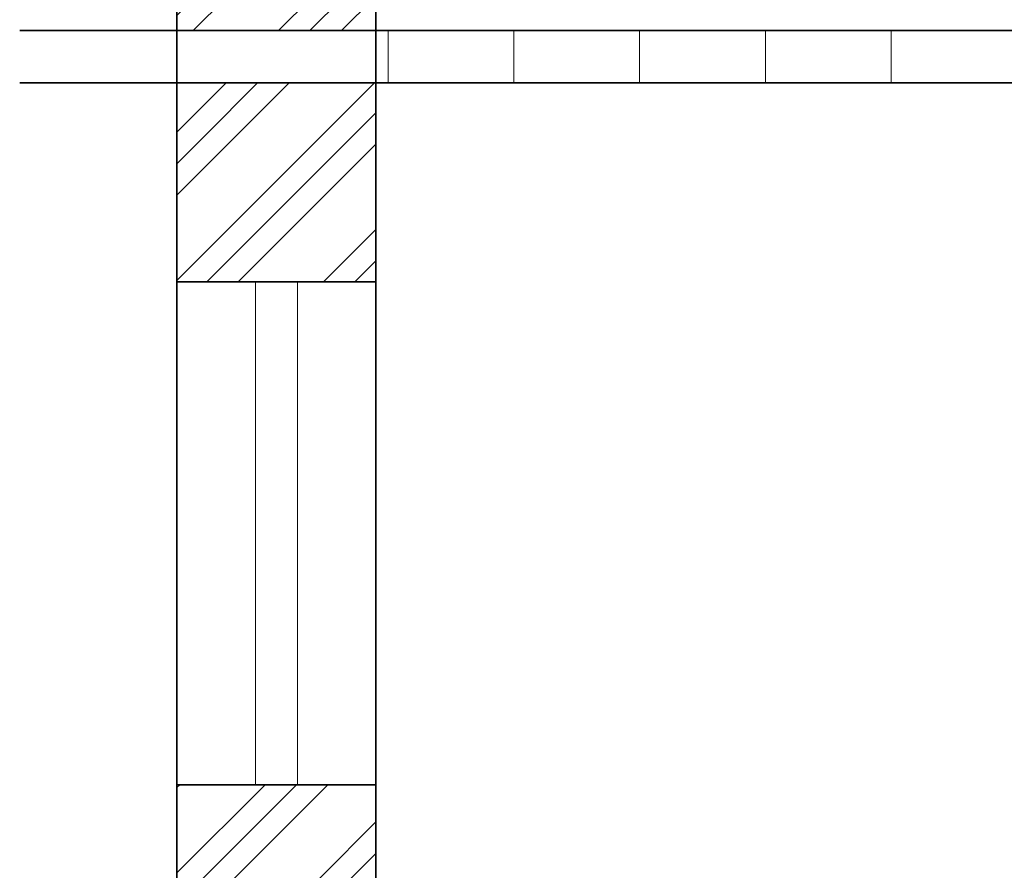
# Model space of a CAD drawing. Units: inches. Extents: x -128 to 854, y -395 to 398.
# Tile 10 of 61: x -71 to 23, y -282 to -201. Entities that reach past the tile are written whole.
import ezdxf

# ---------------------------------------------------------------- set-up
doc = ezdxf.new("R2010")
doc.units = ezdxf.units.IN
doc.header["$MEASUREMENT"] = 0
for name, color, linetype, lineweight in [('A-GLAZ', 220, 'Continuous', 18), ('A-SECT', 220, 'Continuous', 35), ('A-SECT-PATT', 8, 'Continuous', 13)]:
    doc.layers.add(name, color=color, linetype=linetype, lineweight=lineweight)
pattern_1 = [(45, (0, 0), (14.14214, -9e-16), [20]), (45, (3, 0), (14.14214, -9e-16), [20]), (45, (6, 0), (14.14214, -9e-16), [20])]

msp = doc.modelspace()

# ---------------------------------------------------------------- hatches: boundary and pattern name
at = {"layer": 'A-SECT-PATT'}
h = msp.add_hatch(dxfattribs=at)
h.set_pattern_fill('GOST_GROUND', color=256)
h.set_pattern_definition(pattern_1)
h.paths.add_polyline_path([(-37.161, -178.019), (-56.161, -178.019), (-56.161, -202.019), (-37.161, -202.019)])
h.paths.add_polyline_path([(160.839, -178.019), (141.839, -178.019), (141.839, -202.019), (160.839, -202.019)])
h.paths.add_polyline_path([(160.839, -207.019), (141.839, -207.019), (141.839, -226.019), (160.839, -226.019)])
h.paths.add_polyline_path([(317.839, -178.019), (298.839, -178.019), (298.839, -202.019), (317.839, -202.019)])
h.paths.add_polyline_path([(317.839, -207.019), (298.839, -207.019), (298.839, -226.019), (317.839, -226.019)])
h.paths.add_polyline_path([(317.839, -274.019), (298.839, -274.019), (298.839, -298.019), (303.839, -298.019), (312.839, -298.019), (317.839, -298.019)])
h = msp.add_hatch(dxfattribs=at)
h.set_pattern_fill('ANSI31', color=256, scale=96, angle=45, style=0)
h.paths.add_polyline_path([(-38.361, -202.019), (300.039, -202.019), (300.039, -207.019), (-38.361, -207.019)])
h = msp.add_hatch(dxfattribs=at)
h.set_pattern_fill('GOST_GROUND', color=256)
h.set_pattern_definition(pattern_1)
h.paths.add_polyline_path([(-27.161, -322.019), (-37.161, -322.019), (-37.161, -298.019), (-56.161, -298.019), (-56.161, -322.019), (-66.161, -322.019), (-66.161, -346.019), (-27.161, -346.019)])
h.paths.add_polyline_path([(170.839, -322.019), (160.839, -322.019), (160.839, -298.019), (155.839, -298.019), (141.839, -298.019), (141.839, -322.019), (131.839, -322.019), (131.839, -346.019), (170.839, -346.019)])
h.paths.add_polyline_path([(327.839, -322.019), (317.839, -322.019), (317.839, -298.019), (312.839, -298.019), (298.839, -298.019), (298.839, -322.019), (288.839, -322.019), (288.839, -346.019), (327.839, -346.019)])
h.paths.add_polyline_path([(-37.161, -274.019), (-56.161, -274.019), (-56.161, -298.019), (-37.161, -298.019)])
h.paths.add_polyline_path([(-37.161, -207.019), (-56.161, -207.019), (-56.161, -226.019), (-37.161, -226.019)])
h.paths.add_polyline_path([(160.839, -274.019), (141.839, -274.019), (141.839, -298.019), (155.839, -298.019), (160.839, -298.019)])

# ---------------------------------------------------------------- linework, layer by layer
at = {"layer": 'A-GLAZ'}
for p, q in [((-48.661, -226.019), (-48.661, -274.019)), ((-44.661, -226.019), (-44.661, -274.019))]:
    msp.add_line(p, q, dxfattribs=at)
at = {"layer": 'A-SECT'}
for p, q in [((-56.161, -298.019), (-56.161, -178.019)), ((-37.161, -298.019), (-37.161, -178.019)), ((-71.161, -202.019), (-56.161, -202.019)), ((-56.161, -202.019), (317.839, -202.019)), ((-66.161, -207.019), (-71.161, -207.019)), ((-56.161, -207.019), (-66.161, -207.019)), ((-56.161, -207.019), (317.839, -207.019)), ((-56.161, -226.019), (-37.161, -226.019)), ((-56.161, -274.019), (-37.161, -274.019))]:
    msp.add_line(p, q, dxfattribs=at)

doc.saveas('drawing.dxf')
